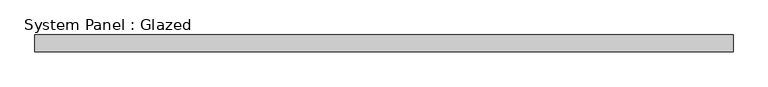
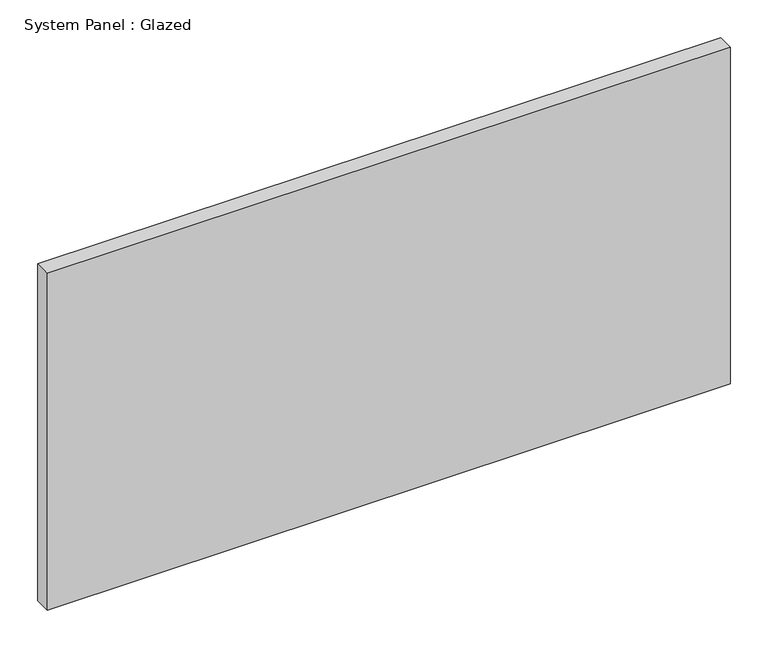
"""IFC4 building model written with IfcOpenShell, lengths in millimetres: plate geometry, System Panel : Glazed."""

from ifc_helpers import new_model, si_unit, origin, origin_with_axes, place, context, project, spatial, polyline, outline, extrude, source, transform, mapped, element, save


def system_panel_glazed_30b75583(model_context):
    return source(origin(), model_context, "Body", "SweptSolid", [
        extrude(outline(polyline([(523.875, 19.05), (-523.875, 19.05), (-523.875, 44.45), (523.875, 44.45), (523.875, 19.05)])), origin_with_axes(), (0.0, 0.0, 1.0), 546.1),
    ])


if __name__ == "__main__":
    model = new_model("IFC4")
    model_context = context("Model", 3, world=origin())
    ifc_project = project(units=[si_unit("LENGTHUNIT", "METRE", prefix="MILLI")], contexts=[model_context])
    site = spatial("IfcSite", under=ifc_project)
    building = spatial("IfcBuilding", under=site)
    placement = place(None, origin())
    system_panel_glazed_shape = system_panel_glazed_30b75583(model_context)
    element("IfcPlate", 1, ObjectType="System Panel : Glazed", at=placement, inside=building, context=model_context, shape_type="MappedRepresentation", body=[
        mapped(system_panel_glazed_shape, transform((0.0, 0.0, 0.0), x_axis=(1.0, 0.0, 0.0), y_axis=(0.0, 1.0, 0.0), z_axis=(0.0, 0.0, 1.0))),
    ])
    save(model, "model.ifc")

# Revit data of these elements
# Type "System Panel : Glazed"
#   Construction Type Id = "GSP4R"
#   Analytic Construction = "1/8 in Pilkington single glazing"
#   Visual Light Transmittance = 0.9
#   Solar Heat Gain Coefficient = 0.86
#   Heat Transfer Coefficient (U) = 1.18115 BTU/(h·ft²·°F)
# Element 1 (IfcPlate, "System Panel : Glazed")
#   Materials on its faces: "Glass"
# Materials
#   "Glass": class "Glass", colour RGB 0 128 192, transparency 0.75, Description = "Soda Lime Glass", Cost = 0
